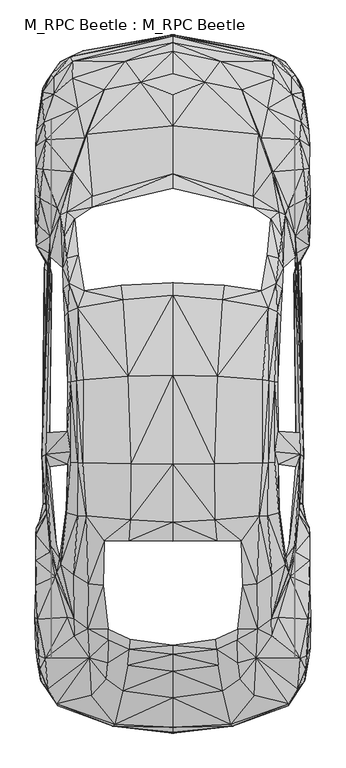
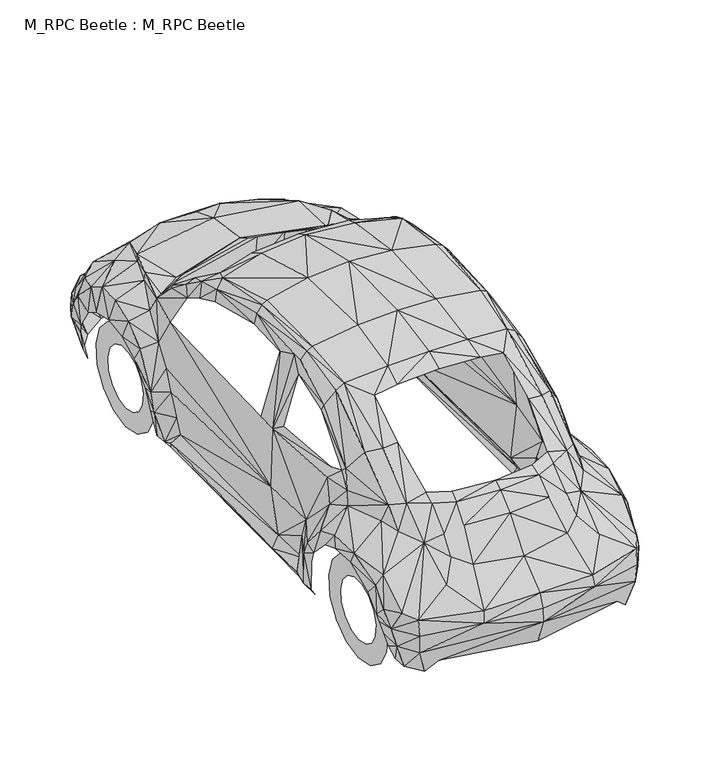
"""IFC4 building model written with IfcOpenShell, lengths in millimetres: proxy geometry, M_RPC Beetle : M_RPC Beetle."""

from ifc_helpers import new_model, si_unit, origin, place, context, project, spatial, triangles, source, transform, mapped, element, save


def m_rpc_beetle_m_rpc_beetle_aa710b07(model_context):
    return source(origin(), model_context, "Body", "Tessellation", [
        triangles([(0.0, -749.071574, 521.742899), (0.0, -720.6335569, 604.0334066), (0.0, -697.1470545, 283.3282547), (0.0, -553.0728908, 738.9057701), (0.0, -753.760096, 438.7513078), (0.0, -253.8386302, 1040.4185434), (0.0, -401.3744104, 922.0218458), (0.0, -305.0182643, 1012.9445663), (0.0, 339.5469707, 1396.6602436), (0.0, 448.9171117, 1443.1075539), (0.0, 778.6050184, 1505.0664173), (0.0, 1285.8879353, 1510.4998066), (0.0, 1742.2541199, 1403.2767002), (0.0, 2432.6093651, 967.8556761), (0.0, 3132.1224815, 632.4714237), (0.0, 3003.4724854, 772.0322365), (0.0, 2706.0784286, 929.3833151), (0.0, 3166.3445206, 220.3177475), (0.0, 2885.1195351, 859.3180424), (0.0, 3224.7104347, 396.0724085), (0.0, 3181.1549538, 556.1401817), (0.0, 3216.1220055, 530.6379956), (-338.407687, -715.988855, 523.3641664), (-331.2653541, -702.6242638, 593.8676027), (-244.8997318, -218.1706584, 1034.7659815), (-249.1500901, -276.1420835, 1003.6112698), (-257.9137267, -368.4231514, 912.4695219), (-249.2377301, 343.0524253, 1381.9373051), (-285.431542, -511.8838351, 760.9462852), (-240.2988317, 460.3974792, 1427.552108), (-236.6180971, 781.4093531, 1494.4185207), (-652.9344915, -590.6250681, 370.7455024), (-540.4532759, -593.7361427, 283.6349946), (-181.3633847, 2956.2803078, 806.8676828), (-253.3566284, 1279.4466133, 1497.179108), (-380.1225826, -444.6667534, 798.8051662), (-371.1837024, -353.5687892, 889.7717068), (-368.2478714, -222.3771967, 1004.1371098), (-368.6422151, -160.8126769, 1037.3951088), (-390.4198465, 343.0962453, 1359.9405373), (-282.758631, 1714.4295101, 1400.2533382), (-397.6060358, 87.5486986, 1216.1732225), (-463.4209139, -538.1308886, 705.2972111), (-271.6726253, 3074.4140854, 663.1441154), (-476.0843851, -323.2904411, 850.4229458), (-464.0343939, 3087.9975586, 214.4022838), (-482.5694544, 95.8303334, 1204.2108713), (-485.3738254, -159.4104914, 1005.7583771), (-569.1103566, 3073.5815781, 547.1136251), (-493.874542, 483.577278, 1392.2346416), (-583.6579788, 3101.4935371, 522.4001627), (-510.6130915, 3134.4011215, 369.6500387), (-392.1287539, 2913.6012268, 783.2935404), (-656.7905062, -598.249421, 480.4223834), (-660.6903408, -585.2354261, 576.6470695), (-562.669071, -200.2052034, 880.3069502), (-560.43436, -101.5266881, 987.8367239), (-512.8039824, 786.711355, 1449.4173431), (-542.1621832, 485.1109054, 1360.7731899), (-564.3779783, 148.6750366, 1173.0999796), (-608.8972449, -561.6174273, 218.6088221), (-511.6209151, 1259.3779255, 1457.1731197), (-542.7756269, 785.2215477, 1431.62715), (-459.1705556, 2305.6242382, 949.6711029), (-601.4481357, -92.8068715, 893.8029287), (-504.0841659, 1766.4854897, 1321.8626289), (-546.4125415, 1253.8568962, 1442.4940739), (-603.419963, 501.4988949, 1279.4466133), (-580.5468678, 789.4280497, 1379.6588104), (-607.6265013, 520.2092717, 1235.979063), (-601.6672357, 965.9276688, 1337.9439148), (-712.9653477, -503.4269022, 590.8879881), (-543.0385468, 1671.1809872, 1362.0876446), (-490.9387473, 2659.6751564, 894.1096687), (-600.0459683, 778.6050184, 1308.1913704), (-598.468521, 1244.567347, 1344.6919041), (-640.0081003, 208.2677382, 1063.2039986), (-680.8904886, -470.5194632, 218.8279221), (-538.8319722, 1968.0490585, 1181.3815962), (-581.3794115, 1249.0805889, 1402.7071129), (-644.9596149, 243.4537263, 1028.9820322), (-502.6819985, 2637.5907486, 866.5918716), (-661.1722881, 162.3463042, 955.8933249), (-690.7057325, -396.8611321, 226.9780968), (-559.5141764, 2176.4921494, 1011.8490664), (-670.6370447, 140.9630437, 873.2960409), (-662.9250154, 324.5173285, 1010.140159), (-615.5138105, 1624.5585423, 1262.9710201), (-595.0507064, 1647.2125374, 1322.1692963), (-589.8363444, 1810.8295853, 1270.2885967), (-729.3095535, -482.3065707, 373.4622334), (-752.0950087, -454.7449173, 476.8731088), (-694.5179272, 315.5346282, 958.4347395), (-727.0748062, -327.5407994, 736.0575428), (-623.3572271, 1778.4478409, 1193.6068674), (-565.035242, 2447.3759056, 934.772957), (-732.2891682, -394.1444012, 324.3420485), (-571.3888876, 2445.9300636, 884.7764448), (-699.1188091, 280.0419, 808.1822828), (-604.6907066, 1951.091518, 1171.2596123), (-587.8206971, 3015.1278786, 200.2490234), (-691.4068525, 574.6314222, 283.8102565), (-750.7366613, -381.2618663, 397.2555121), (-627.9581091, 1897.5456585, 1125.469602), (-602.8941593, 2217.067725, 949.8025629), (-619.8517725, 2074.2204849, 1075.9988571), (-710.949773, 550.0056361, 448.9171117), (-765.2404272, -360.5796985, 467.8465522), (-699.9952091, 763.1372126, 1016.187101), (-763.8382599, -313.4313409, 671.381912), (-758.3609779, -391.2085702, 565.035242), (-717.9606823, 496.6350929, 583.9646825), (-723.2188643, 461.5367266, 181.1004829), (-718.1358896, 554.8256181, 180.0050192), (-771.9884165, -342.0446016, 511.3579951), (-574.3247186, 2977.4883156, 683.0814159), (-731.2813808, 376.1351443, 185.3070212), (-541.5487032, 2807.2984131, 783.4688204), (-640.1833803, 2199.9349045, 944.8949409), (-739.4315374, 551.9336071, 222.5524585), (-782.1104731, -268.9559124, 609.6421486), (-772.8209965, -106.1275973, 756.4329706), (-722.2110043, 958.3909195, 967.6803961), (-703.8074038, 810.6798775, 292.5300731), (-725.3220789, 835.6124399, 965.0074488), (-758.2733379, 370.7893224, 225.6197313), (-785.878775, -90.0025096, 695.9639145), (-780.1824657, 80.9759712, 676.0266867), (-779.9195457, 89.5643278, 755.1622633), (-760.9024652, 444.4038334, 223.2973804), (-778.6050184, 192.2302905, 631.3321037), (-659.0690735, 2238.6700401, 850.3353058), (-771.4626492, 345.7253363, 426.4822165), (-774.7051838, 315.3593482, 502.0247349), (-781.7160931, 232.4115588, 696.3582945), (-719.7134096, 810.6360575, 185.964303), (-690.3551725, 1860.1249775, 294.1075386), (-697.1470545, 1960.2056419, 957.0763922), (-780.2701057, 377.6249516, 532.7412466), (-778.6488384, 417.28038, 440.0220151), (-746.0042467, 820.1446341, 614.0677505), (-678.173794, 2886.7845497, 671.0752447), (-698.0233818, 2078.8215122, 757.3970106), (-640.0519203, 3071.2590454, 391.9535102), (-713.4911877, 1919.5424263, 537.0792449), (-718.6617296, 1911.1731697, 193.1066541), (-705.6477711, 1983.2978371, 648.7279169), (-731.2813808, 1892.3751892, 233.5070043), (-674.4492393, 2909.8328522, 198.8030179), (-727.3815462, 2040.3052586, 190.0832013), (-722.1233643, 1974.7094078, 190.0832013), (-678.6557413, 2984.5867195, 540.8914395), (-700.0828491, 2817.5957497, 206.339749), (-696.8403145, 2993.6132034, 517.7554607), (-724.1390116, 2626.4609047, 788.1135223), (-699.5570091, 1883.7430126, 390.6389465), (-765.4157072, 2043.5477932, 362.8144094), (-742.2797647, 2459.3382568, 809.2338902), (-716.6460823, 2967.1470863, 449.8372953), (-766.9493345, 2002.4901249, 376.836228), (-732.0700682, 2726.2786491, 728.1264862), (-771.6817492, 2086.0075562, 482.5694544), (-759.6317579, 2292.960767, 780.6206657), (-769.5346418, 2144.7677776, 699.5131891), (-778.0791784, 2024.2239727, 495.1452856), (-742.9808121, 2848.794136, 602.2806793), (-782.6362404, 2187.1399006, 616.8721579), (-740.0450174, 2920.3932541, 427.6652839), (-741.6224648, 2898.4841263, 520.1654517), (-750.9119413, 2806.3345184, 398.3509395), (-782.7677004, 2314.7385075, 681.1972286), (-778.6050184, 2464.4649788, 693.9920872), (-760.4204453, 2788.5004326, 455.533641), (-774.7051838, 2684.6515388, 603.069403), (-780.8835131, 2591.1871857, 666.7810301), (-743.1122721, 809.6720901, 220.5368294), (0.0, 2350.6693085, 1011.8490664), (-459.1705556, 2241.4745201, 1007.2920044), (0.0, 1813.2394672, 1369.1424465), (-294.1513586, 1797.0267941, 1360.0720699), (-580.6345078, 850.2914858, 1382.7260651), (338.407687, -715.988855, 523.3641664), (331.2653541, -702.6242638, 593.8676027), (244.8997318, -218.1706584, 1034.7659815), (249.1500901, -276.1420835, 1003.6112698), (257.9137267, -368.4231514, 912.4695219), (249.2377301, 343.0524253, 1381.9373051), (285.431542, -511.8838351, 760.9462852), (240.2988317, 460.3974792, 1427.552108), (236.6180971, 781.4093531, 1494.4185207), (652.9344915, -590.6250681, 370.7455024), (540.4532759, -593.7361427, 283.6349946), (181.3633847, 2956.2803078, 806.8676828), (253.3566284, 1279.4466133, 1497.179108), (380.1225826, -444.6667534, 798.8051662), (371.1837024, -353.5687892, 889.7717068), (368.2478714, -222.3771967, 1004.1371098), (368.6422151, -160.8126769, 1037.3951088), (390.4198465, 343.0962453, 1359.9405373), (282.758631, 1714.4295101, 1400.2533382), (397.6060358, 87.5486986, 1216.1732225), (463.4209139, -538.1308886, 705.2972111), (271.6726253, 3074.4140854, 663.1441154), (476.0843851, -323.2904411, 850.4229458), (464.0343939, 3087.9975586, 214.4022838), (482.5694544, 95.8303334, 1204.2108713), (485.3738254, -159.4104914, 1005.7583771), (569.1103566, 3073.5815781, 547.1136251), (493.874542, 483.577278, 1392.2346416), (583.6579788, 3101.4935371, 522.4001627), (510.6130915, 3134.4011215, 369.6500387), (392.1287539, 2913.6012268, 783.2935404), (656.7905062, -598.249421, 480.4223834), (660.6903408, -585.2354261, 576.6470695), (562.669071, -200.2052034, 880.3069502), (560.43436, -101.5266881, 987.8367239), (512.8039824, 786.711355, 1449.4173431), (542.1621832, 485.1109054, 1360.7731899), (564.3779783, 148.6750366, 1173.0999796), (608.8972449, -561.6174273, 218.6088221), (511.6209151, 1259.3779255, 1457.1731197), (542.7756269, 785.2215477, 1431.62715), (459.1705556, 2305.6242382, 949.6711029), (601.4481357, -92.8068715, 893.8029287), (504.0841659, 1766.4854897, 1321.8626289), (546.4125415, 1253.8568962, 1442.4940739), (603.419963, 501.4988949, 1279.4466133), (580.5468678, 789.4280497, 1379.6588104), (607.6265013, 520.2092717, 1235.979063), (601.6672357, 965.9276688, 1337.9439148), (712.9653477, -503.4269022, 590.8879881), (543.0385468, 1671.1809872, 1362.0876446), (490.9387473, 2659.6751564, 894.1096687), (600.0459683, 778.6050184, 1308.1913704), (598.468521, 1244.567347, 1344.6919041), (640.0081003, 208.2677382, 1063.2039986), (680.9343086, -470.5194632, 218.8279221), (538.8319722, 1968.0490585, 1181.3815962), (581.3794115, 1249.0805889, 1402.7071129), (644.9596149, 243.4537263, 1028.9820322), (502.6819985, 2637.5907486, 866.5918716), (661.1722881, 162.3463042, 955.8933249), (690.7057325, -396.8611321, 226.9780968), (559.5141764, 2176.4921494, 1011.8490664), (670.6370447, 140.9630437, 873.2960409), (662.9250154, 324.5173285, 1010.140159), (615.5138105, 1624.5585423, 1262.9710201), (595.0507064, 1647.2125374, 1322.1692963), (589.8363444, 1810.8295853, 1270.2885967), (729.3095535, -482.3065707, 373.4622334), (752.0950087, -454.7449173, 476.8731088), (694.5179272, 315.5346282, 958.4347395), (727.0748062, -327.5407994, 736.0575428), (623.3572271, 1778.4478409, 1193.6068674), (565.035242, 2447.3759056, 934.772957), (732.2891682, -394.1444012, 324.3420485), (571.3888876, 2445.9300636, 884.7764448), (699.1188091, 280.0419, 808.1822828), (604.6907066, 1951.091518, 1171.2596123), (587.8206971, 3015.1278786, 200.2490234), (691.4068525, 574.6314222, 283.8102565), (750.7366613, -381.2618663, 397.2555121), (627.9581091, 1897.5456585, 1125.469602), (602.8941593, 2217.067725, 949.8025629), (619.8517725, 2074.2204849, 1075.9988571), (710.949773, 550.0056361, 448.9171117), (765.2404272, -360.5796985, 467.8465522), (699.9952091, 763.1372126, 1016.187101), (763.8382599, -313.4313409, 671.381912), (758.3609779, -391.2085702, 565.035242), (717.9606823, 496.6350929, 583.9646825), (723.2188643, 461.5367266, 181.1004829), (718.1358896, 554.8256181, 180.0050192), (771.9884165, -342.0446016, 511.3579951), (574.3247186, 2977.4883156, 683.0814159), (731.2813808, 376.1351443, 185.3070212), (541.5487032, 2807.2984131, 783.4688204), (640.1833803, 2199.9349045, 944.8949409), (739.4315374, 551.9336071, 222.5524585), (782.1104731, -268.9559124, 609.6421486), (772.8209965, -106.1275973, 756.4329706), (722.2548243, 958.3909195, 967.6803961), (703.8074038, 810.6798775, 292.5300731), (725.3220789, 835.6124399, 965.0074488), (758.2733379, 370.7893224, 225.6197313), (785.878775, -90.0025096, 695.9639145), (780.1824657, 80.9759712, 676.0266867), (779.9633657, 89.5643278, 755.1622633), (760.9024652, 444.4038334, 223.2973804), (778.6050184, 192.2302905, 631.3321037), (659.0690735, 2238.6700401, 850.3353058), (771.4626492, 345.7253363, 426.4822165), (774.7051838, 315.3593482, 502.0247349), (781.7160931, 232.4115588, 696.3582945), (719.7134096, 810.6360575, 185.964303), (690.3551725, 1860.1249775, 294.1075386), (697.1470545, 1960.2056419, 957.0763922), (780.2701057, 377.6249516, 532.7412466), (778.6488384, 417.28038, 440.0220151), (746.0042467, 820.1446341, 614.0677505), (678.173794, 2886.7845497, 671.0752447), (698.0233818, 2078.8215122, 757.3970106), (640.0519203, 3071.2590454, 391.9535102), (713.4911877, 1919.5424263, 537.0792449), (718.6617296, 1911.1731697, 193.1066541), (705.6477711, 1983.2978371, 648.7279169), (731.2813808, 1892.3751892, 233.5070043), (674.4492393, 2909.8328522, 198.8030179), (727.3815462, 2040.3052586, 190.0832013), (722.1233643, 1974.7094078, 190.0832013), (678.6557413, 2984.5867195, 540.8914395), (700.0828491, 2817.5957497, 206.339749), (696.8403145, 2993.6132034, 517.7554607), (724.1390116, 2626.4609047, 788.1135223), (699.5570091, 1883.7430126, 390.6389465), (765.4157072, 2043.5477932, 362.8144094), (742.2797647, 2459.3382568, 809.2338902), (716.6460823, 2967.1470863, 449.8372953), (766.9493345, 2002.4901249, 376.836228), (732.0700682, 2726.2786491, 728.1264862), (771.7255692, 2086.0075562, 482.5694544), (759.6317579, 2292.960767, 780.6206657), (769.5346418, 2144.7677776, 699.5131891), (778.0791784, 2024.2239727, 495.1452856), (742.9808121, 2848.794136, 602.2806793), (782.6362404, 2187.1399006, 616.8721579), (740.0450174, 2920.3932541, 427.6652839), (741.6224648, 2898.4841263, 520.1654517), (750.9119413, 2806.3345184, 398.3509395), (782.7677004, 2314.7385075, 681.1972286), (778.6050184, 2464.4649788, 693.9920872), (760.4204453, 2788.5004326, 455.533641), (774.7051838, 2684.6515388, 603.069403), (780.8835131, 2591.1871857, 666.7810301), (743.1122721, 809.6720901, 220.5368294), (459.1705556, 2241.4745201, 1007.2920044), (294.1513586, 1797.0267941, 1360.0720699), (580.6345078, 850.2914858, 1382.7260651), (-693.6415998, 2431.9082451, 0.0015117), (-693.6415998, 2431.9082451, 117.9161946), (-693.6415998, 2558.849334, 26.9935013), (-693.6415998, 2509.4663017, 134.3918241), (-693.6415998, 2663.794091, 103.2371124), (-693.6415998, 2573.6600578, 181.0143508), (-693.6415998, 2728.6886765, 215.6307153), (-693.6415998, 2613.3154861, 249.7212399), (-693.6415998, 2742.2721497, 344.6752187), (-693.6415998, 2621.5969574, 328.5939328), (-693.6415998, 2702.1786667, 468.1109982), (-693.6415998, 2597.102813, 404.0049911), (-693.6415998, 2615.3310608, 564.5109644), (-693.6415998, 2544.0389008, 462.94042), (-693.6415998, 2496.8028305, 617.3118113), (-693.6415998, 2471.5636734, 495.2344153), (-693.6415998, 2367.0135143, 617.3118113), (-693.6415998, 2392.2528168, 495.2344153), (-693.6415998, 2248.4854294, 564.5109644), (-693.6415998, 2319.7775894, 462.94042), (-693.6415998, 2161.6378235, 468.1109982), (-693.6415998, 2266.7136772, 404.0049911), (-693.6415998, 2121.5441952, 344.6752187), (-693.6415998, 2242.2193874, 328.5939328), (-693.6415998, 2135.1278137, 215.6307153), (-693.6415998, 2250.501004, 249.7212399), (-693.6415998, 2200.0225445, 103.2371124), (-693.6415998, 2290.1564323, 181.0143508), (-693.6415998, 2304.9670109, 26.9935013), (-693.6415998, 2354.3500431, 134.3918241), (693.6415998, 2431.9082451, 0.0015117), (693.6415998, 2431.9082451, 117.9161946), (693.6415998, 2304.9670109, 26.9935013), (693.6415998, 2354.3500431, 134.3918241), (693.6415998, 2200.0225445, 103.2371124), (693.6415998, 2290.1564323, 181.0143508), (693.6415998, 2135.1278137, 215.6307153), (693.6415998, 2250.501004, 249.7212399), (693.6415998, 2121.5441952, 344.6752187), (693.6415998, 2242.2193874, 328.5939328), (693.6415998, 2161.6378235, 468.1109982), (693.6415998, 2266.7136772, 404.0049911), (693.6415998, 2248.4854294, 564.5109644), (693.6415998, 2319.7775894, 462.94042), (693.6415998, 2367.0135143, 617.3118113), (693.6415998, 2392.2528168, 495.2344153), (693.6415998, 2496.8028305, 617.3118113), (693.6415998, 2471.5636734, 495.2344153), (693.6415998, 2615.3310608, 564.5109644), (693.6415998, 2544.0389008, 462.94042), (693.6415998, 2702.1786667, 468.1109982), (693.6415998, 2597.102813, 404.0049911), (693.6415998, 2742.2721497, 344.6752187), (693.6415998, 2621.5969574, 328.5939328), (693.6415998, 2728.6886765, 215.6307153), (693.6415998, 2613.3154861, 249.7212399), (693.6415998, 2663.794091, 103.2371124), (693.6415998, 2573.6600578, 181.0143508), (693.6415998, 2558.849334, 26.9935013), (693.6415998, 2509.4663017, 134.3918241), (-693.6415998, -13.583631, 0.0015117), (-693.6415998, -13.583631, 117.9161946), (-693.6415998, 113.3575975, 26.9935013), (-693.6415998, 63.9745244, 134.3918241), (-693.6415998, 218.3021002, 103.2371124), (-693.6415998, 128.1681397, 181.0143508), (-693.6415998, 283.1968128, 215.6307153), (-693.6415998, 167.823568, 249.7212399), (-693.6415998, 296.7804314, 344.6752187), (-693.6415998, 176.1052028, 328.5939328), (-693.6415998, 256.6868212, 468.1109982), (-693.6415998, 151.6108585, 404.0049911), (-693.6415998, 169.8392153, 564.5109644), (-693.6415998, 98.5470553, 462.94042), (-693.6415998, 51.3110713, 617.3118113), (-693.6415998, 26.0718098, 495.2344153), (-693.6415998, -78.4783311, 617.3118113), (-693.6415998, -53.2390741, 495.2344153), (-693.6415998, -197.0064706, 564.5109644), (-693.6415998, -125.7143196, 462.94042), (-693.6415998, -283.8540765, 468.1109982), (-693.6415998, -178.7781137, 404.0049911), (-693.6415998, -323.9477048, 344.6752187), (-693.6415998, -203.2724762, 328.5939328), (-693.6415998, -310.3640862, 215.6307153), (-693.6415998, -194.9908414, 249.7212399), (-693.6415998, -245.4693737, 103.2371124), (-693.6415998, -155.335395, 181.0143508), (-693.6415998, -140.5248618, 26.9935013), (-693.6415998, -91.1417842, 134.3918241), (693.6415998, -13.583631, 0.0015117), (693.6415998, -13.583631, 117.9161946), (693.6415998, -140.5248618, 26.9935013), (693.6415998, -91.1417842, 134.3918241), (693.6415998, -245.4693737, 103.2371124), (693.6415998, -155.335395, 181.0143508), (693.6415998, -310.3640862, 215.6307153), (693.6415998, -194.9908414, 249.7212399), (693.6415998, -323.9477048, 344.6752187), (693.6415998, -203.2724762, 328.5939328), (693.6415998, -283.8540765, 468.1109982), (693.6415998, -178.7781137, 404.0049911), (693.6415998, -197.0064706, 564.5109644), (693.6415998, -125.7143196, 462.94042), (693.6415998, -78.4783311, 617.3118113), (693.6415998, -53.2390741, 495.2344153), (693.6415998, 51.3110713, 617.3118113), (693.6415998, 26.0718098, 495.2344153), (693.6415998, 169.8392153, 564.5109644), (693.6415998, 98.5470553, 462.94042), (693.6415998, 256.6868212, 468.1109982), (693.6415998, 151.6108585, 404.0049911), (693.6415998, 296.7804314, 344.6752187), (693.6415998, 176.1052028, 328.5939328), (693.6415998, 283.1968128, 215.6307153), (693.6415998, 167.823568, 249.7212399), (693.6415998, 218.3021002, 103.2371124), (693.6415998, 128.1681397, 181.0143508), (693.6415998, 113.3575975, 26.9935013), (693.6415998, 63.9745244, 134.3918241)], [[67, 58, 62], [67, 63, 58], [53, 82, 74], [34, 17, 19], [118, 82, 53], [155, 98, 82], [155, 158, 98], [34, 74, 17], [172, 155, 175], [172, 158, 155], [159, 168, 169], [166, 142, 169], [175, 161, 174], [175, 155, 161], [142, 152, 169], [154, 169, 152], [160, 145, 165], [160, 156, 145], [162, 160, 165], [162, 157, 160], [34, 53, 74], [74, 96, 64], [82, 96, 74], [82, 98, 96], [36, 29, 27], [29, 43, 24], [23, 55, 54], [23, 24, 55], [23, 2, 24], [23, 1, 2], [5, 1, 23], [134, 140, 133], [134, 139, 140], [117, 130, 113], [117, 126, 130], [113, 120, 114], [113, 130, 120], [140, 112, 107], [140, 139, 112], [92, 108, 103], [91, 103, 97], [91, 92, 103], [61, 33, 32], [84, 78, 91], [84, 91, 97], [38, 26, 25], [77, 81, 83], [63, 50, 58], [63, 59, 50], [68, 63, 69], [68, 59, 63], [181, 75, 69], [74, 64, 17], [64, 14, 17], [64, 178, 14], [178, 177, 14], [34, 19, 16], [53, 34, 44], [21, 44, 15], [21, 49, 44], [44, 34, 15], [34, 16, 15], [22, 49, 21], [22, 51, 49], [20, 51, 22], [20, 52, 51], [18, 52, 20], [18, 46, 52], [51, 152, 49], [51, 154, 152], [101, 144, 46], [144, 52, 46], [101, 159, 144], [159, 169, 154], [101, 168, 159], [101, 149, 168], [149, 170, 168], [149, 153, 170], [168, 173, 169], [168, 170, 173], [49, 142, 116], [49, 152, 142], [49, 116, 44], [116, 142, 118], [161, 155, 118], [155, 82, 118], [142, 161, 118], [158, 132, 98], [158, 163, 132], [172, 163, 158], [172, 171, 163], [98, 119, 96], [98, 132, 119], [171, 164, 163], [171, 167, 164], [163, 143, 132], [163, 164, 143], [96, 105, 64], [96, 119, 105], [105, 178, 64], [105, 85, 178], [167, 165, 164], [167, 162, 165], [165, 143, 164], [165, 147, 143], [150, 160, 157], [150, 151, 160], [151, 156, 160], [151, 148, 137], [13, 35, 12], [13, 41, 35], [12, 31, 11], [12, 35, 31], [35, 58, 31], [35, 62, 58], [11, 30, 10], [11, 31, 30], [31, 50, 30], [31, 58, 50], [10, 28, 9], [10, 30, 28], [30, 40, 28], [30, 50, 40], [125, 75, 181], [125, 109, 75], [125, 87, 109], [125, 93, 87], [123, 141, 125], [137, 141, 156], [137, 124, 141], [148, 124, 137], [148, 176, 124], [146, 176, 148], [146, 136, 176], [141, 112, 125], [112, 93, 125], [112, 99, 93], [124, 112, 141], [124, 107, 112], [124, 102, 107], [176, 102, 124], [176, 120, 102], [136, 120, 176], [136, 114, 120], [47, 40, 50], [47, 42, 40], [48, 42, 47], [48, 39, 42], [57, 47, 60], [57, 48, 47], [60, 50, 59], [60, 47, 50], [59, 77, 60], [59, 68, 77], [77, 57, 60], [77, 83, 57], [70, 77, 68], [70, 81, 77], [75, 68, 69], [75, 70, 68], [26, 6, 25], [26, 8, 6], [27, 8, 26], [27, 7, 8], [29, 7, 27], [29, 4, 7], [24, 4, 29], [24, 2, 4], [32, 5, 23], [33, 5, 32], [33, 3, 5], [32, 23, 54], [55, 45, 72], [55, 24, 43], [99, 83, 93], [99, 86, 83], [135, 86, 99], [135, 129, 86], [131, 129, 135], [131, 128, 129], [93, 81, 87], [93, 83, 81], [128, 122, 129], [128, 127, 122], [122, 86, 129], [122, 65, 86], [86, 57, 83], [86, 65, 57], [127, 110, 122], [127, 121, 110], [110, 94, 122], [122, 94, 65], [94, 56, 65], [56, 57, 65], [56, 48, 57], [56, 45, 48], [94, 45, 56], [115, 110, 121], [115, 111, 110], [111, 94, 110], [111, 72, 94], [108, 92, 115], [92, 111, 115], [78, 32, 91], [78, 61, 32], [45, 38, 48], [45, 37, 38], [37, 26, 38], [37, 27, 26], [36, 27, 37], [134, 135, 139], [134, 131, 135], [139, 99, 112], [139, 135, 99], [126, 140, 130], [126, 133, 140], [130, 107, 120], [130, 140, 107], [120, 107, 102], [45, 36, 37], [92, 55, 72], [92, 54, 55], [91, 54, 92], [91, 32, 54], [92, 72, 111], [72, 45, 94], [43, 45, 55], [43, 36, 45], [43, 29, 36], [79, 90, 66], [79, 100, 90], [90, 73, 66], [85, 100, 79], [85, 106, 100], [85, 105, 106], [105, 119, 106], [95, 88, 89], [90, 89, 73], [89, 67, 73], [73, 67, 62], [89, 76, 80], [89, 80, 67], [88, 76, 89], [73, 35, 41], [73, 62, 35], [69, 63, 181], [80, 63, 67], [76, 71, 80], [146, 148, 151], [141, 147, 145], [151, 137, 156], [173, 166, 169], [173, 174, 166], [166, 174, 161], [166, 161, 142], [52, 144, 51], [144, 154, 51], [144, 159, 154], [116, 53, 44], [116, 118, 53], [119, 143, 138], [143, 119, 132], [143, 147, 138], [138, 104, 119], [119, 104, 106], [104, 100, 106], [104, 90, 100], [104, 95, 90], [95, 89, 90], [25, 39, 38], [38, 39, 48], [141, 138, 147], [156, 141, 145], [165, 145, 147], [41, 179, 180], [41, 13, 179], [66, 41, 180], [66, 73, 41], [123, 125, 71], [125, 181, 71], [71, 181, 80], [181, 63, 80], [138, 141, 123], [226, 221, 217], [226, 217, 222], [212, 233, 241], [193, 19, 17], [277, 212, 241], [314, 241, 257], [314, 257, 317], [193, 17, 233], [331, 334, 314], [331, 314, 317], [318, 328, 327], [325, 328, 301], [334, 333, 320], [334, 320, 314], [301, 328, 311], [313, 311, 328], [319, 324, 304], [319, 304, 315], [321, 324, 319], [321, 319, 316], [193, 233, 212], [233, 223, 255], [241, 233, 255], [241, 255, 257], [195, 186, 188], [188, 183, 202], [182, 213, 214], [182, 214, 183], [182, 183, 2], [182, 2, 1], [5, 182, 1], [293, 292, 299], [293, 299, 298], [276, 272, 289], [276, 289, 285], [272, 273, 279], [272, 279, 289], [299, 266, 271], [299, 271, 298], [251, 262, 267], [250, 256, 262], [250, 262, 251], [220, 191, 192], [243, 250, 237], [243, 256, 250], [197, 184, 185], [236, 242, 240], [222, 217, 209], [222, 209, 218], [227, 228, 222], [227, 222, 218], [338, 228, 234], [233, 17, 223], [223, 17, 14], [223, 14, 336], [336, 14, 177], [193, 16, 19], [212, 203, 193], [21, 15, 203], [21, 203, 208], [203, 15, 193], [193, 15, 16], [22, 21, 208], [22, 208, 210], [20, 22, 210], [20, 210, 211], [18, 20, 211], [18, 211, 205], [210, 208, 311], [210, 311, 313], [260, 205, 303], [303, 205, 211], [260, 303, 318], [318, 313, 328], [260, 318, 327], [260, 327, 308], [308, 327, 329], [308, 329, 312], [327, 328, 332], [327, 332, 329], [208, 275, 301], [208, 301, 311], [208, 203, 275], [275, 277, 301], [320, 277, 314], [314, 277, 241], [301, 277, 320], [317, 257, 291], [317, 291, 322], [331, 317, 322], [331, 322, 330], [257, 255, 278], [257, 278, 291], [330, 322, 323], [330, 323, 326], [322, 291, 302], [322, 302, 323], [255, 223, 264], [255, 264, 278], [264, 223, 336], [264, 336, 244], [326, 323, 324], [326, 324, 321], [324, 323, 302], [324, 302, 306], [309, 316, 319], [309, 319, 310], [310, 319, 315], [310, 296, 307], [13, 12, 194], [13, 194, 200], [12, 11, 190], [12, 190, 194], [194, 190, 217], [194, 217, 221], [11, 10, 189], [11, 189, 190], [190, 189, 209], [190, 209, 217], [10, 9, 187], [10, 187, 189], [189, 187, 199], [189, 199, 209], [284, 338, 234], [284, 234, 268], [284, 268, 246], [284, 246, 252], [282, 284, 300], [296, 315, 300], [296, 300, 283], [307, 296, 283], [307, 283, 335], [305, 307, 335], [305, 335, 295], [300, 284, 271], [271, 284, 252], [271, 252, 258], [283, 300, 271], [283, 271, 266], [283, 266, 261], [335, 283, 261], [335, 261, 279], [295, 335, 279], [295, 279, 273], [206, 209, 199], [206, 199, 201], [207, 206, 201], [207, 201, 198], [216, 219, 206], [216, 206, 207], [219, 218, 209], [219, 209, 206], [218, 219, 236], [218, 236, 227], [236, 219, 216], [236, 216, 242], [229, 227, 236], [229, 236, 240], [234, 228, 227], [234, 227, 229], [185, 184, 6], [185, 6, 8], [186, 185, 8], [186, 8, 7], [188, 186, 7], [188, 7, 4], [183, 188, 4], [183, 4, 2], [191, 182, 5], [192, 191, 5], [192, 5, 3], [191, 213, 182], [214, 231, 204], [214, 202, 183], [258, 252, 242], [258, 242, 245], [294, 258, 245], [294, 245, 288], [290, 294, 288], [290, 288, 287], [252, 246, 240], [252, 240, 242], [287, 288, 281], [287, 281, 286], [281, 288, 245], [281, 245, 224], [245, 242, 216], [245, 216, 224], [286, 281, 269], [286, 269, 280], [269, 281, 253], [281, 224, 253], [253, 224, 215], [215, 224, 216], [215, 216, 207], [215, 207, 204], [253, 215, 204], [274, 280, 269], [274, 269, 270], [270, 269, 253], [270, 253, 231], [267, 274, 251], [251, 274, 270], [237, 250, 191], [237, 191, 220], [204, 207, 197], [204, 197, 196], [196, 197, 185], [196, 185, 186], [195, 196, 186], [293, 298, 294], [293, 294, 290], [298, 271, 258], [298, 258, 294], [285, 289, 299], [285, 299, 292], [289, 279, 266], [289, 266, 299], [279, 261, 266], [204, 196, 195], [251, 231, 214], [251, 214, 213], [250, 251, 213], [250, 213, 191], [251, 270, 231], [231, 253, 204], [202, 214, 204], [202, 204, 195], [202, 195, 188], [238, 225, 249], [238, 249, 259], [249, 225, 232], [244, 238, 259], [244, 259, 265], [244, 265, 264], [264, 265, 278], [254, 248, 247], [249, 232, 248], [248, 232, 226], [232, 221, 226], [248, 239, 235], [248, 226, 239], [247, 248, 235], [232, 200, 194], [232, 194, 221], [228, 338, 222], [239, 226, 222], [235, 239, 230], [305, 310, 307], [300, 304, 306], [310, 315, 296], [332, 328, 325], [332, 325, 333], [325, 320, 333], [325, 301, 320], [211, 210, 303], [303, 210, 313], [303, 313, 318], [275, 203, 212], [275, 212, 277], [278, 297, 302], [302, 291, 278], [302, 297, 306], [297, 278, 263], [278, 265, 263], [263, 265, 259], [263, 259, 249], [263, 249, 254], [254, 249, 248], [184, 197, 198], [197, 207, 198], [300, 306, 297], [315, 304, 300], [324, 306, 304], [200, 337, 179], [200, 179, 13], [225, 337, 200], [225, 200, 232], [282, 230, 284], [284, 230, 338], [230, 239, 338], [338, 239, 222], [297, 282, 300], [339, 342, 341], [339, 340, 342], [341, 344, 343], [341, 342, 344], [343, 346, 345], [343, 344, 346], [345, 348, 347], [345, 346, 348], [347, 350, 349], [347, 348, 350], [349, 352, 351], [349, 350, 352], [351, 354, 353], [351, 352, 354], [353, 356, 355], [353, 354, 356], [355, 358, 357], [355, 356, 358], [357, 360, 359], [357, 358, 360], [359, 362, 361], [359, 360, 362], [361, 364, 363], [361, 362, 364], [363, 366, 365], [363, 364, 366], [365, 368, 367], [365, 366, 368], [367, 340, 339], [367, 368, 340], [369, 372, 371], [369, 370, 372], [371, 374, 373], [371, 372, 374], [373, 376, 375], [373, 374, 376], [375, 378, 377], [375, 376, 378], [377, 380, 379], [377, 378, 380], [379, 382, 381], [379, 380, 382], [381, 384, 383], [381, 382, 384], [383, 386, 385], [383, 384, 386], [385, 388, 387], [385, 386, 388], [387, 390, 389], [387, 388, 390], [389, 392, 391], [389, 390, 392], [391, 394, 393], [391, 392, 394], [393, 396, 395], [393, 394, 396], [395, 398, 397], [395, 396, 398], [397, 370, 369], [397, 398, 370], [399, 402, 401], [399, 400, 402], [401, 404, 403], [401, 402, 404], [403, 406, 405], [403, 404, 406], [405, 408, 407], [405, 406, 408], [407, 410, 409], [407, 408, 410], [409, 412, 411], [409, 410, 412], [411, 414, 413], [411, 412, 414], [413, 416, 415], [413, 414, 416], [415, 418, 417], [415, 416, 418], [417, 420, 419], [417, 418, 420], [419, 422, 421], [419, 420, 422], [421, 424, 423], [421, 422, 424], [423, 426, 425], [423, 424, 426], [425, 428, 427], [425, 426, 428], [427, 400, 399], [427, 428, 400], [429, 432, 431], [429, 430, 432], [431, 434, 433], [431, 432, 434], [433, 436, 435], [433, 434, 436], [435, 438, 437], [435, 436, 438], [437, 440, 439], [437, 438, 440], [439, 442, 441], [439, 440, 442], [441, 444, 443], [441, 442, 444], [443, 446, 445], [443, 444, 446], [445, 448, 447], [445, 446, 448], [447, 450, 449], [447, 448, 450], [449, 452, 451], [449, 450, 452], [451, 454, 453], [451, 452, 454], [453, 456, 455], [453, 454, 456], [455, 458, 457], [455, 456, 458], [457, 430, 429], [457, 458, 430]], closed=False),
    ])


if __name__ == "__main__":
    model = new_model("IFC4")
    model_context = context("Model", 3, world=origin())
    ifc_project = project(units=[si_unit("LENGTHUNIT", "METRE", prefix="MILLI")], contexts=[model_context])
    site = spatial("IfcSite", under=ifc_project)
    building = spatial("IfcBuilding", under=site)
    placement = place(None, origin())
    m_rpc_beetle_m_rpc_beetle_shape = m_rpc_beetle_m_rpc_beetle_aa710b07(model_context)
    element("IfcBuildingElementProxy", 1, Name="M_RPC Beetle : M_RPC Beetle", ObjectType="M_RPC Beetle : M_RPC Beetle", at=placement, inside=building, context=model_context, shape_type="MappedRepresentation", body=[
        mapped(m_rpc_beetle_m_rpc_beetle_shape, transform((0.0, 0.0, 0.0), x_axis=(1.0, 0.0, 0.0), y_axis=(0.0, 1.0, 0.0), z_axis=(0.0, 0.0, 1.0))),
    ])
    save(model, "model.ifc")

# Revit data of these elements
# Type "M_RPC Beetle : M_RPC Beetle"
#   built-in parameter 1005198 = "{2, 15},{39, RPC-16-0U6E-L4EG-ENH1-J3KF-SVEL-0TX4-C0},{1, 0},{1, 0},{2, 45},{1, 8},{5, Color},{1, 0},{1, 0},{3, 0.8},{3, 0.8},{3, 0.8},{1, 8},{7, BBoxMin},{1, 0},{1, 0},{1, 0},{1, 0},{1, 0},{1, 8},{7, BBoxMax},{1, 0},{1, 0},{1, 0},{1, 0},{1, 0},{2, 11},{9, RPCTypeId},{1, 0},{1, 0},{39, RPC-16-0U6E-L4EG-ENH1-J3KF-SVEL-0TX4-C0},{1, 6},{14, RPCPlantHeight},{1, 0},{1, 0},{4, 4.92},{2, 11},{7, keyword},{1, 0},{1, 0},{27, :Geometry:RPC:VW Beetle [4]},{2, 11},{8, category},{1, 0},{1, 0},{21, :Auto_Economy/Midsize},{2, 11},{12, LocalizedUID},{1, 0},{1, 0},{13, VW Beetle [4]},{2, 14},{6, Height},{1, 0},{1, 0},{4, 4.92},{1, 2},{16, Cast Reflections},{1, 0},{1, 0},{1, 0},{1, 4},{12, Transparency},{1, 0},{1, 0},{2, 18},{1, 4},{7, Tinting},{1, 0},{1, 0},{2, 50},{1, 2},{11, Use Tinting},{1, 0},{1, 0},{1, 0},{1, 2},{13, License Plate},{1, 0},{1, 0},{1, 0},{2, 11},{21, License Plate Texture},{1, 0},{1, 0},{64, __RPC:/object data/textures/car/plate/textures/default/rgb/0/0/0},{2, 11},{23, i_License Plate Texture},{1, 0},{1, 0},{0, },{1, 2},{12, Custom Plate},{1, 0},{1, 0},{1, 0},{2, 11},{23, License Plate File Name},{1, 0},{1, 0},{0, },{2, 11},{20, AdvancedUIDefinition},{1, 0},{1, 0},{0, },{2, 11},{10, AssetLibID},{1, 0},{1, 0},{36, 4D3F6E72-3F99-4203-98E9-AF80B3C7A7A4},{2, 11},{10, BaseSchema},{1, 0},{1, 0},{9, RPCSchema},{2, 11},{12, ExchangeGUID},{1, 0},{1, 0},{0, },{1, 2},{6, Hidden},{1, 0},{1, 0},{1, 0},{1, 4},{11, RPCCategory},{1, 0},{1, 0},{1, 0},{2, 11},{8, RPCImage},{1, 0},{1, 0},{0, },{1, 4},{13, SchemaVersion},{1, 0},{1, 0},{1, 4},{2, 11},{12, UIDefinition},{1, 0},{1, 0},{0, },{2, 11},{6, UIName},{1, 0},{1, 0},{39, RPC-16-0U6E-L4EG-ENH1-J3KF-SVEL-0TX4-C0},{2, 11},{11, VersionGUID},{1, 0},{1, 0},{9, RPCSchema},{2, 11},{9, assettype},{1, 0},{1, 0},{11, RPCGeometry},{2, 11},{11, description},{1, 0},{1, 0},{0, },{2, 11},{9, localname},{1, 0},{1, 0},{3, RPC},{2, 11},{9, localtype},{1, 0},{1, 0},{3, RPC},{1, 4},{8, revision},{1, 0},{1, 0},{1, 1},{2, 11},{9, thumbnail},{1, 0},{1, 0},{0, },{1, 4},{7, version},{1, 0},{1, 0},{1, 1},{1, 2},{20, RPC_Cast Reflections},{1, 0},{1, 0},{1, 1},{1, 4},{16, RPC_Transparency},{1, 0},{1, 0},{2, 18},{1, 4},{11, RPC_Tinting},{1, 0},{1, 0},{2, 50},{1, 2},{15, RPC_Use Tinting},{1, 0},{1, 0},{1, 0},{1, 2},{17, RPC_License Plate},{1, 0},{1, 0},{1, 0},{2, 11},{25, RPC_License Plate Texture},{1, 0},{1, 0},{64, __RPC:/object data/textures/car/plate/textures/default/rgb/0/0/0},{2, 11},{27, RPC_i_License Plate Texture},{1, 0},{1, 0},{0, },{1, 2},{16, RPC_Custom Plate},{1, 0},{1, 0},{1, 0},{2, 11},{27, RPC_License Plate File Name},{1, 0},{1, 0},{0, },{21, assetlibrary_base.fbx},{1, 5},"
#   built-in parameter 1005195 = "RPC-16-0U6E-L4EG-ENH1-J3KF-SVEL-0TX4-C0"
#   Height = 0
